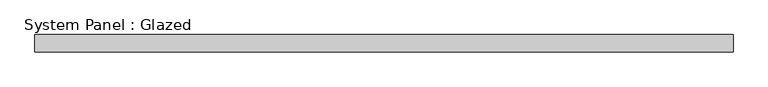
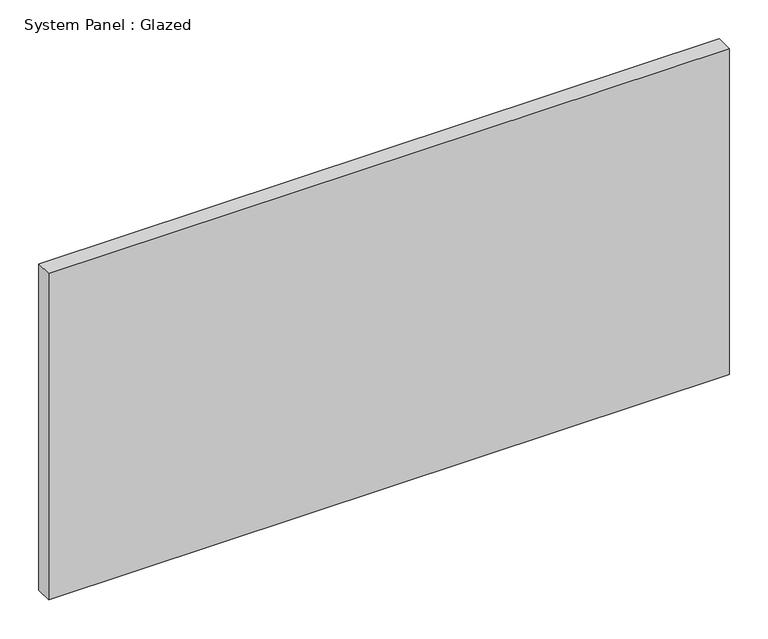
"""IFC4 building model written with IfcOpenShell, lengths in millimetres: plate geometry, System Panel : Glazed."""

from ifc_helpers import new_model, si_unit, origin, origin_with_axes, place, context, project, spatial, polyline, outline, extrude, source, transform, mapped, element, save


def system_panel_glazed_c5c5478c(model_context):
    return source(origin(), model_context, "Body", "SweptSolid", [
        extrude(outline(polyline([(507.2023702, 19.05), (-507.2023702, 19.05), (-507.2023702, 44.45), (507.2023702, 44.45), (507.2023702, 19.05)])), origin_with_axes(), (0.0, 0.0, 1.0), 514.35),
    ])


if __name__ == "__main__":
    model = new_model("IFC4")
    model_context = context("Model", 3, world=origin())
    ifc_project = project(units=[si_unit("LENGTHUNIT", "METRE", prefix="MILLI")], contexts=[model_context])
    site = spatial("IfcSite", under=ifc_project)
    building = spatial("IfcBuilding", under=site)
    placement = place(None, origin())
    system_panel_glazed_shape = system_panel_glazed_c5c5478c(model_context)
    element("IfcPlate", 1, ObjectType="System Panel : Glazed", at=placement, inside=building, context=model_context, shape_type="MappedRepresentation", body=[
        mapped(system_panel_glazed_shape, transform((0.0, 0.0, 0.0), x_axis=(1.0, 0.0, 0.0), y_axis=(0.0, 1.0, 0.0), z_axis=(0.0, 0.0, 1.0))),
    ])
    save(model, "model.ifc")

# Revit data of these elements
# Type "System Panel : Glazed"
#   Construction Type Id = "GSP4R"
#   Analytic Construction = "1/8 in Pilkington single glazing"
#   Visual Light Transmittance = 0.9
#   Solar Heat Gain Coefficient = 0.86
#   Heat Transfer Coefficient (U) = 1.18115 BTU/(h·ft²·°F)
#   Define Thermal Properties by = 1
# Element 1 (IfcPlate, "System Panel : Glazed")
#   Materials on its faces: "Glass"
# Materials
#   "Glass": class "Glass", colour RGB 0 128 192, transparency 0.75, Description = "Soda Lime Glass", Cost = 0
